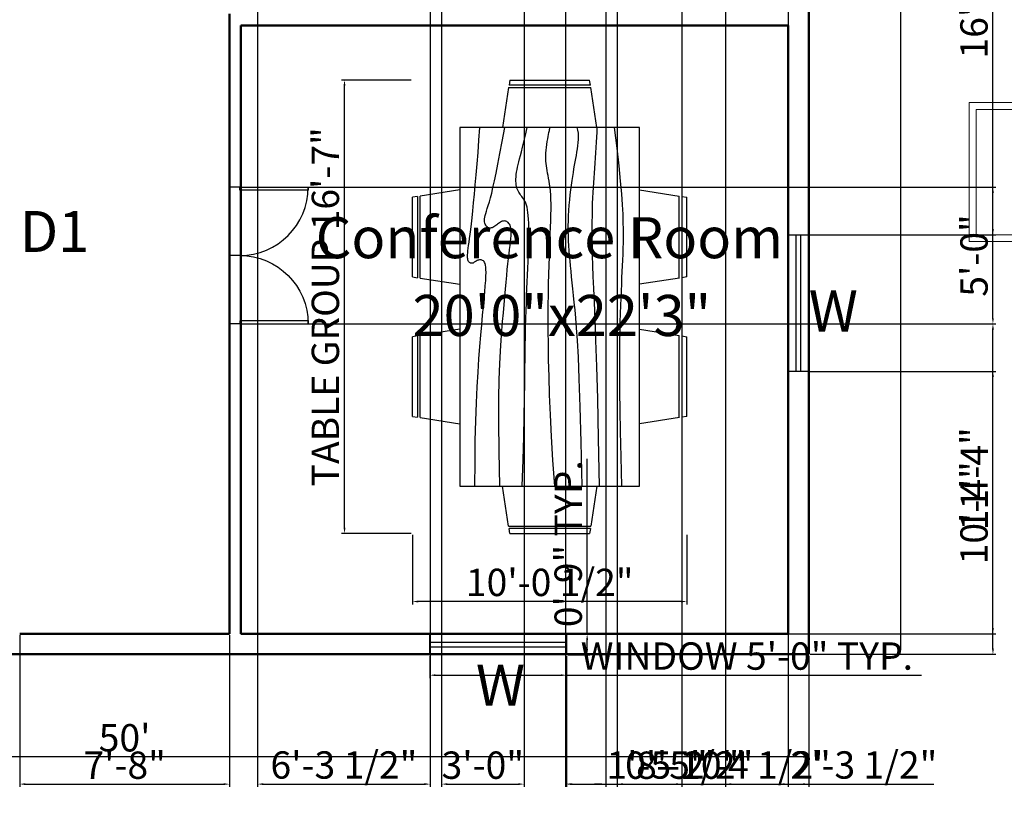
# Model space of a CAD drawing. Units: inches. Extents: x 1953 to 3378, y 1378 to 2530.
# Tile 2 of 5: x 2350 to 2782, y 1378 to 1725. Entities that reach past the tile are written whole.
import ezdxf

# ---------------------------------------------------------------- set-up
doc = ezdxf.new("R2010")
doc.units = ezdxf.units.IN
for name, color, linetype, lineweight in [('A-ANNO-DIMS', 2, 'Continuous', 18), ('A-ANNO-TEXT', 7, 'Continuous', 18), ('A-AREA-IDEN', 4, 'Continuous', 18), ('A-DOOR', 4, 'Continuous', 25), ('A-FURN', 50, 'Continuous', 25), ('wall', 7, 'Continuous', 50), ('windows', 180, 'Continuous', 25)]:
    doc.layers.add(name, color=color, linetype=linetype, lineweight=lineweight)
doc.styles.get("Standard").update_dxf_attribs({"font": 'arial.ttf'})
doc.dimstyles.new('ISO-25', dxfattribs={"dimtxt": 12, "dimasz": 2.5, "dimexe": 1.25, "dimexo": 0.625, "dimtad": 1, "dimdec": 1, "dimlunit": 4, "dimtxsty": 'Standard', "dimcen": 2.5, "dimadec": 0, "dimazin": 0, "dimtfac": 1, "dimtdec": 1, "dimtmove": 0, "dimatfit": 3, "dimfxl": 1, "dimarcsym": 0})

# ---------------------------------------------------------------- blocks, each defined once
blk = doc.blocks.new('*U2')
for p, q in [((0, 0), (0, -6)), ((40, 0), (40, -6))]:
    blk.add_line(p, q)
blk.add_lwpolyline([(0, 0), (0, 40), (1.75, 40), (1.75, 0)], close=True)
blk.add_arc((0, 0), 40, 0, 90)
blk = doc.blocks.new('Dining Set - 36 x 72 in.')
for p, q in [((-22.2343, 26.00059), (-23.4847, 17.99762)), ((-22.2304, 26), (-5.7608, 26)), ((-22, 27.5), (-22.1562, 26.50042)), ((-5.8416, 26.5), (-22.1534, 26.5)), ((-22, 27.5), (-6, 27.5)), ((-5.8437, 26.49966), (-6, 27.5)), ((-4.5152, 17.99762), (-5.7655, 25.99926)), ((5.7657, 26.00059), (4.5153, 17.99762)), ((5.7696, 26), (22.2392, 26)), ((6, 27.5), (5.8438, 26.50042)), ((22.1584, 26.5), (5.8466, 26.5)), ((6, 27.5), (22, 27.5)), ((22.1563, 26.49966), (22, 27.5)), ((23.4848, 17.99762), (22.2345, 25.99926)), ((36, 18), (-36, 18)), ((-36, 18), (-36, -18)), ((36, -18), (36, 18)), ((-45.5, 8), (-44.5004, 8.15617)), ((-45.5, 8), (-45.5, -8)), ((-44.5, -8.15843), (-44.5, 8.15338)), ((-44.0006, 8.23428), (-35.9976, 9.48474)), ((-44, 8.23041), (-44, -8.23915)), ((44.0006, 8.23428), (35.9976, 9.48474)), ((44, 8.23041), (44, -8.23915)), ((44.5, -8.15843), (44.5, 8.15338)), ((45.5, 8), (44.5005, 8.15617)), ((45.5, 8), (45.5, -8)), ((-44.4997, -8.15631), (-45.5, -8)), ((-35.9976, -9.48476), (-43.9993, -8.2345)), ((35.9976, -9.48476), (43.9993, -8.2345)), ((44.4997, -8.15631), (45.5, -8)), ((-36, -18), (36, -18)), ((-22.2343, -26.0006), (-23.4847, -17.99762)), ((-4.5152, -17.99762), (-5.7655, -25.99928)), ((5.7657, -26.0006), (4.5153, -17.99762)), ((23.4848, -17.99762), (22.2345, -25.99928)), ((-22.2304, -26), (-5.7608, -26)), ((-22, -27.5), (-22.1562, -26.50044)), ((-5.8416, -26.5), (-22.1534, -26.5)), ((-22, -27.5), (-6, -27.5)), ((-5.8437, -26.49967), (-6, -27.5)), ((5.7696, -26), (22.2392, -26)), ((6, -27.5), (5.8438, -26.50044)), ((22.1584, -26.5), (5.8466, -26.5)), ((6, -27.5), (22, -27.5)), ((22.1563, -26.49967), (22, -27.5))]:
    blk.add_line(p, q)
for points in [[(-36, 15), (-31.1772, 14.97754), (-26.8079, 14.91406), (-22.8538, 14.81543), (-19.276, 14.6875), (-16.0362, 14.53613), (-13.0957, 14.36718), (-10.4159, 14.18652), (-7.9583, 14), (-5.6904, 13.81315), (-3.6035, 13.63021), (-1.6954, 13.45508), (0.0365, 13.29166), (1.5945, 13.14388), (2.9811, 13.01562), (4.1988, 12.9108), (5.25, 12.83333), (6.1393, 12.78613), (6.8802, 12.76823), (7.4883, 12.77767), (7.9792, 12.8125), (8.3685, 12.87077), (8.6719, 12.95052), (8.9049, 13.0498), (9.0833, 13.16666), (9.2205, 13.29899), (9.3216, 13.44401), (9.3895, 13.59879), (9.4271, 13.76041), (9.4373, 13.92594), (9.4232, 14.09245), (9.3875, 14.257), (9.3333, 14.41666), (9.2638, 14.56917), (9.1836, 14.71484), (9.0975, 14.85465), (9.0104, 14.98958), (8.9272, 15.1206), (8.8529, 15.2487), (8.7922, 15.37483), (8.75, 15.5), (8.7305, 15.62467), (8.7344, 15.74739), (8.7617, 15.86621), (8.8125, 15.97916), (8.8867, 16.08431), (8.9844, 16.17968), (9.1055, 16.26334), (9.25, 16.33333), (9.4189, 16.38802), (9.6172, 16.42708), (9.8506, 16.45052), (10.125, 16.45833), (10.4463, 16.45052), (10.8203, 16.42708), (11.2529, 16.38802), (11.75, 16.33333), (12.3184, 16.26318), (12.9694, 16.17838), (13.7151, 16.07991), (14.5677, 15.96875), (15.5395, 15.84586), (16.6426, 15.71224), (17.8893, 15.56884), (19.2917, 15.41666), (20.859, 15.25667), (22.5879, 15.08984), (24.4721, 14.91715), (26.5052, 14.73958), (28.6809, 14.5581), (30.9929, 14.3737), (33.4347, 14.18733), (36, 14)], [(-36, 10), (-28.9766, 10.14274), (-23.1725, 10.20442), (-18.4241, 10.19775), (-14.5677, 10.13541), (-11.4399, 10.03011), (-8.877, 9.89453), (-6.7154, 9.74137), (-4.7917, 9.58333), (-2.9698, 9.43082), (-1.2246, 9.28515), (0.4415, 9.14534), (2.026, 9.01041), (3.5266, 8.87939), (4.9408, 8.7513), (6.266, 8.62516), (7.5, 8.5), (8.6411, 8.37549), (9.6914, 8.2539), (10.6538, 8.13818), (11.5312, 8.03125), (12.3267, 7.93603), (13.043, 7.85547), (13.6831, 7.79248), (14.25, 7.75), (14.7471, 7.7303), (15.1797, 7.73307), (15.5537, 7.75732), (15.875, 7.80208), (16.1494, 7.86637), (16.3828, 7.94922), (16.5811, 8.04964), (16.75, 8.16666), (16.8944, 8.29915), (17.0143, 8.44531), (17.1089, 8.60319), (17.1771, 8.77083), (17.218, 8.94629), (17.2305, 9.1276), (17.2137, 9.31282), (17.1667, 9.5), (17.0895, 9.6875), (16.987, 9.875), (16.8649, 10.0625), (16.7292, 10.25), (16.5856, 10.4375), (16.4401, 10.625), (16.2985, 10.8125), (16.1667, 11), (16.05, 11.18733), (15.9518, 11.3737), (15.8752, 11.5581), (15.8229, 11.73958), (15.798, 11.91715), (15.8034, 12.08984), (15.842, 12.25667), (15.9167, 12.41666), (16.0295, 12.56836), (16.1784, 12.70833), (16.3605, 12.83268), (16.5729, 12.9375), (16.8127, 13.01888), (17.0768, 13.07291), (17.3625, 13.0957), (17.6667, 13.08333), (17.9894, 13.03312), (18.3418, 12.94726), (18.7382, 12.82918), (19.1927, 12.68229), (19.7195, 12.51001), (20.3327, 12.31575), (21.0465, 12.10294), (21.875, 11.875), (22.8357, 11.63354), (23.959, 11.37304), (25.2786, 11.08618), (26.8282, 10.76562), (28.6414, 10.40405), (30.752, 9.99414), (33.1936, 9.52856), (36, 9)], [(-36, 5.5), (-30.7157, 5.3348), (-26.069, 5.20963), (-21.9946, 5.11767), (-18.4271, 5.05208), (-15.3009, 5.00602), (-12.5508, 4.97265), (-10.1112, 4.94515), (-7.9167, 4.91666), (-5.909, 4.88167), (-4.0586, 4.83984), (-2.3429, 4.79215), (-0.7396, 4.73958), (0.7739, 4.6831), (2.22, 4.6237), (3.6213, 4.56233), (5, 4.5), (6.373, 4.43782), (7.7344, 4.3776), (9.0723, 4.32129), (10.375, 4.27083), (11.6309, 4.22819), (12.8281, 4.19531), (13.9551, 4.17415), (15, 4.16666), (15.954, 4.17448), (16.819, 4.19791), (17.6001, 4.23698), (18.3021, 4.29166), (18.9299, 4.36198), (19.4883, 4.44791), (19.9823, 4.54948), (20.4167, 4.66666), (20.7969, 4.79899), (21.1302, 4.94401), (21.4245, 5.09879), (21.6875, 5.26041), (21.9271, 5.42594), (22.1511, 5.59245), (22.3672, 5.757), (22.5834, 5.91666), (22.8065, 6.06868), (23.0404, 6.21093), (23.2879, 6.34147), (23.5521, 6.45833), (23.8358, 6.55957), (24.142, 6.64323), (24.4735, 6.70735), (24.8334, 6.75), (25.2235, 6.76969), (25.642, 6.76692), (26.0858, 6.74267), (26.5521, 6.69791), (27.0379, 6.63362), (27.5404, 6.55078), (28.0565, 6.45036), (28.5834, 6.33333), (29.1242, 6.19987), (29.7071, 6.04687), (30.3661, 5.87044), (31.1354, 5.66666), (32.0493, 5.43164), (33.142, 5.16146), (34.4475, 4.85221), (36, 4.5)], [(-36, -1), (-30.7915, -0.6591), (-26.0195, -0.38216), (-21.6519, -0.16284), (-17.6563, 0.00521), (-14.0005, 0.12833), (-10.6523, 0.21289), (-7.5796, 0.26522), (-4.75, 0.29166), (-2.134, 0.29793), (0.2878, 0.28711), (2.5317, 0.26163), (4.6146, 0.22396), (6.5529, 0.17651), (8.3633, 0.12174), (10.0623, 0.06209), (11.6667, 0), (13.1899, -0.06201), (14.6341, -0.1211), (15.9982, -0.17432), (17.2813, -0.21875), (18.4823, -0.25147), (19.6003, -0.26953), (20.6343, -0.27002), (21.5834, -0.25), (22.4481, -0.20768), (23.2357, -0.14584), (23.9549, -0.06836), (24.6146, 0.02083), (25.2235, 0.11784), (25.7904, 0.21875), (26.3241, 0.31966), (26.8334, 0.41666), (27.3265, 0.50618), (27.8099, 0.58593), (28.2894, 0.65397), (28.7709, 0.70833), (29.2601, 0.74707), (29.763, 0.76823), (30.2855, 0.76985), (30.8334, 0.75), (31.4088, 0.70784), (31.9994, 0.64713), (32.589, 0.57275), (33.1615, 0.48958), (33.7008, 0.4025), (34.1908, 0.3164), (34.6153, 0.23616), (34.9584, 0.16666), (35.2099, 0.11165), (35.3848, 0.07031), (35.504, 0.04069), (35.5886, 0.02083), (35.6594, 0.00879), (35.7377, 0.0026), (35.8442, 0.00032), (36, 0)], [(-36, -6.5), (-27.1843, -6.31267), (-20.084, -6.1263), (-14.469, -5.9419), (-10.1094, -5.76042), (-6.7752, -5.58285), (-4.2363, -5.41016), (-2.2629, -5.24333), (-0.625, -5.08334), (0.8708, -4.93099), (2.2715, -4.78646), (3.5872, -4.64974), (4.8281, -4.52084), (6.0046, -4.39974), (7.127, -4.28646), (8.2053, -4.18099), (9.25, -4.08334), (10.2705, -3.99382), (11.2734, -3.91407), (12.2647, -3.84603), (13.25, -3.79167), (14.2354, -3.75293), (15.2266, -3.73177), (16.2295, -3.73015), (17.25, -3.75), (18.2912, -3.79248), (19.3451, -3.85547), (20.4009, -3.93604), (21.4479, -4.03125), (22.4754, -4.13819), (23.4727, -4.25391), (24.4289, -4.37549), (25.3334, -4.5), (26.1785, -4.62492), (26.9694, -4.74935), (27.7145, -4.87281), (28.4219, -4.99479), (29.1, -5.11483), (29.7572, -5.23242), (30.4016, -5.34709), (31.0417, -5.45834), (31.6837, -5.56437), (32.3262, -5.65821), (32.9658, -5.73153), (33.599, -5.77604), (34.2224, -5.78345), (34.8327, -5.74545), (35.4264, -5.65373), (36, -5.5)], [(-36, -10), (-26.4022, -9.81299), (-18.4675, -9.62891), (-11.9839, -9.45069), (-6.7396, -9.28125), (-2.5226, -9.12354), (0.8789, -8.98047), (3.6769, -8.85498), (6.0833, -8.75), (8.2767, -8.66765), (10.3021, -8.60677), (12.1712, -8.56543), (13.8958, -8.54167), (15.4876, -8.53353), (16.9583, -8.53907), (18.3197, -8.55632), (19.5834, -8.58334), (20.7616, -8.61841), (21.8685, -8.66081), (22.9188, -8.71004), (23.9271, -8.76563), (24.9081, -8.82707), (25.8763, -8.89388), (26.8465, -8.96558), (27.8334, -9.04167), (28.8474, -9.12118), (29.8828, -9.20117), (30.93, -9.27824), (31.9792, -9.34896), (33.0205, -9.40991), (34.0443, -9.45768), (35.0407, -9.48885), (36, -9.5)], [(-36, -14.5), (-30.0881, -14.33513), (-25.0332, -14.21224), (-20.7312, -14.12647), (-17.0781, -14.07292), (-13.97, -14.04671), (-11.3027, -14.04297), (-8.9724, -14.05681), (-6.875, -14.08334), (-4.9224, -14.11833), (-3.0905, -14.16016), (-1.3709, -14.20785), (0.2448, -14.26042), (1.7647, -14.3169), (3.1973, -14.3763), (4.5507, -14.43767), (5.8333, -14.5), (7.0554, -14.5621), (8.235, -14.62175), (9.3922, -14.67652), (10.5469, -14.72396), (11.7192, -14.76164), (12.929, -14.78711), (14.1965, -14.79794), (15.5417, -14.79167), (16.9933, -14.76424), (18.6152, -14.70508), (20.4804, -14.60197), (22.6615, -14.44271), (25.2312, -14.21509), (28.2624, -13.9069), (31.8277, -13.50594), (36, -13)]]:
    blk.add_lwpolyline(points)
blk = doc.blocks.new('*D27')
at = {"layer": 'A-ANNO-DIMS', "color": 0, "lineweight": -2, "transparency": 16777216}
for p, q in [((2696.37, 2286.01), (2737.23, 2286.01)), ((2735.98, 2283.51), (2735.98, 1448.51)), ((2696.37, 1446.01), (2737.23, 1446.01))]:
    blk.add_line(p, q, dxfattribs=at)
at = {"layer": 'A-ANNO-DIMS', "color": 0, "transparency": 16777216}
for points in [[(2735.56, 2283.51), (2736.4, 2283.51), (2735.98, 2286.01)], [(2735.56, 1448.51), (2736.4, 1448.51), (2735.98, 1446.01)]]:
    blk.add_solid(points, dxfattribs=at)
at = {"layer": 'Defpoints', "color": 0, "transparency": 16777216}
for p in [(2695.75, 2286.01), (2695.75, 1446.01), (2735.98, 1446.01)]:
    blk.add_point(p, dxfattribs=at)
at = {"layer": 'A-ANNO-DIMS', "color": 0, "transparency": 16777216, "insert": (2729.23, 1866.01), "char_height": 12, "attachment_point": 5, "rotation": 90}
blk.add_mtext("70'", dxfattribs=at)
blk = doc.blocks.new('*D28')
at = {"layer": 'A-ANNO-DIMS', "color": 0, "lineweight": -2, "transparency": 16777216}
for p, q in [((2095.75, 1445.39), (2095.75, 1399.8)), ((2695.75, 1445.39), (2695.75, 1399.8)), ((2693.25, 1401.05), (2098.25, 1401.05))]:
    blk.add_line(p, q, dxfattribs=at)
at = {"layer": 'A-ANNO-DIMS', "color": 0, "transparency": 16777216}
for points in [[(2098.25, 1401.47), (2098.25, 1400.63), (2095.75, 1401.05)], [(2693.25, 1401.47), (2693.25, 1400.63), (2695.75, 1401.05)]]:
    blk.add_solid(points, dxfattribs=at)
at = {"layer": 'Defpoints', "color": 0, "transparency": 16777216}
for p in [(2095.75, 1446.01), (2695.75, 1446.01), (2095.75, 1401.05)]:
    blk.add_point(p, dxfattribs=at)
at = {"layer": 'A-ANNO-DIMS', "color": 0, "transparency": 16777216, "insert": (2395.75, 1407.8), "char_height": 12, "attachment_point": 5}
blk.add_mtext("50'", dxfattribs=at)
blk = doc.blocks.new('WINDOW-60IN')
for p, q in [((0, 5.5), (60, 5.5)), ((0, 5.5), (60, 5.5)), ((0, 3.5), (60, 3.5))]:
    blk.add_line(p, q)
blk.add_lwpolyline([(0, 9), (60, 9), (60, 0), (0, 0)], close=True)
blk = doc.blocks.new('*D38')
at = {"layer": 'A-ANNO-DIMS', "color": 0, "lineweight": -2, "transparency": 16777216}
for p, q in [((2529.57, 1445.21), (2529.57, 1435.58)), ((2589.57, 1445.21), (2589.57, 1435.58)), ((2532.07, 1436.83), (2587.07, 1436.83)), ((2589.57, 1436.83), (2745.17, 1436.83))]:
    blk.add_line(p, q, dxfattribs=at)
at = {"layer": 'A-ANNO-DIMS', "color": 0, "transparency": 16777216}
for points in [[(2532.07, 1437.25), (2532.07, 1436.42), (2529.57, 1436.83)], [(2587.07, 1437.25), (2587.07, 1436.42), (2589.57, 1436.83)]]:
    blk.add_solid(points, dxfattribs=at)
at = {"layer": 'Defpoints', "color": 0, "transparency": 16777216}
for p in [(2529.57, 1445.83), (2589.57, 1445.83), (2589.57, 1436.83)]:
    blk.add_point(p, dxfattribs=at)
at = {"layer": 'A-ANNO-DIMS', "color": 0, "transparency": 16777216, "insert": (2668.62, 1443.67), "char_height": 12, "attachment_point": 5}
blk.add_mtext('WINDOW 5\'-0" TYP.', dxfattribs=at)
blk = doc.blocks.new('*D39')
at = {"layer": 'A-ANNO-DIMS', "color": 0, "lineweight": -2, "transparency": 16777216}
for p, q in [((2598.57, 1454.83), (2598.57, 1531.73)), ((2590.19, 1454.83), (2599.82, 1454.83)), ((2598.57, 1448.33), (2598.57, 1452.33)), ((2590.19, 1445.83), (2599.82, 1445.83))]:
    blk.add_line(p, q, dxfattribs=at)
at = {"layer": 'A-ANNO-DIMS', "color": 0, "transparency": 16777216}
for points in [[(2598.15, 1452.33), (2598.98, 1452.33), (2598.57, 1454.83)], [(2598.15, 1448.33), (2598.98, 1448.33), (2598.57, 1445.83)]]:
    blk.add_solid(points, dxfattribs=at)
at = {"layer": 'Defpoints', "color": 0, "transparency": 16777216}
for p in [(2589.57, 1454.83), (2598.57, 1454.83), (2589.57, 1445.83)]:
    blk.add_point(p, dxfattribs=at)
at = {"layer": 'A-ANNO-DIMS', "color": 0, "transparency": 16777216, "insert": (2591.82, 1494.53), "char_height": 12, "attachment_point": 5, "rotation": 90}
blk.add_mtext('0\'-9" TYP.', dxfattribs=at)
blk = doc.blocks.new('*D50')
at = {"layer": 'A-ANNO-DIMS', "color": 0, "lineweight": -2, "transparency": 16777216}
for p, q in [((2521.4, 1697.99), (2490.93, 1697.99)), ((2492.18, 1501.51), (2492.18, 1695.49)), ((2521.4, 1499.01), (2490.93, 1499.01))]:
    blk.add_line(p, q, dxfattribs=at)
at = {"layer": 'A-ANNO-DIMS', "color": 0, "transparency": 16777216}
for points in [[(2491.76, 1695.49), (2492.59, 1695.49), (2492.18, 1697.99)], [(2491.76, 1501.51), (2492.59, 1501.51), (2492.18, 1499.01)]]:
    blk.add_solid(points, dxfattribs=at)
at = {"layer": 'Defpoints', "color": 0, "transparency": 16777216}
for p in [(2492.18, 1697.99), (2522.02, 1697.99), (2522.02, 1499.01)]:
    blk.add_point(p, dxfattribs=at)
at = {"layer": 'A-ANNO-DIMS', "color": 0, "transparency": 16777216, "insert": (2485.34, 1598.5), "char_height": 12, "attachment_point": 5, "rotation": 90}
blk.add_mtext('TABLE GROUP 16\'-7"', dxfattribs=at)
blk = doc.blocks.new('*D51')
at = {"layer": 'A-ANNO-DIMS', "color": 0, "lineweight": -2, "transparency": 16777216}
for p, q in [((2522.02, 1498.39), (2522.02, 1467.92)), ((2642.28, 1498.39), (2642.28, 1467.92)), ((2639.78, 1469.17), (2524.52, 1469.17))]:
    blk.add_line(p, q, dxfattribs=at)
at = {"layer": 'A-ANNO-DIMS', "color": 0, "transparency": 16777216}
for points in [[(2524.52, 1469.59), (2524.52, 1468.75), (2522.02, 1469.17)], [(2639.78, 1469.59), (2639.78, 1468.75), (2642.28, 1469.17)]]:
    blk.add_solid(points, dxfattribs=at)
at = {"layer": 'Defpoints', "color": 0, "transparency": 16777216}
for p in [(2522.02, 1499.01), (2642.28, 1499.01), (2522.02, 1469.17)]:
    blk.add_point(p, dxfattribs=at)
at = {"layer": 'A-ANNO-DIMS', "color": 0, "transparency": 16777216, "insert": (2582.15, 1476), "char_height": 12, "attachment_point": 5}
blk.add_mtext('10\'-0 1/2"', dxfattribs=at)
blk = doc.blocks.new('*D70')
at = {"layer": 'A-ANNO-DIMS', "color": 0, "lineweight": -2, "transparency": 16777216}
for p, q in [((2696.37, 1570.16), (2777.76, 1570.16)), ((2776.51, 1448.51), (2776.51, 1567.66)), ((2696.37, 1446.01), (2777.76, 1446.01))]:
    blk.add_line(p, q, dxfattribs=at)
at = {"layer": 'A-ANNO-DIMS', "color": 0, "transparency": 16777216}
for points in [[(2776.09, 1567.66), (2776.93, 1567.66), (2776.51, 1570.16)], [(2776.09, 1448.51), (2776.93, 1448.51), (2776.51, 1446.01)]]:
    blk.add_solid(points, dxfattribs=at)
at = {"layer": 'Defpoints', "color": 0, "transparency": 16777216}
for p in [(2695.75, 1570.16), (2776.51, 1570.16), (2695.75, 1446.01)]:
    blk.add_point(p, dxfattribs=at)
at = {"layer": 'A-ANNO-DIMS', "color": 0, "transparency": 16777216, "insert": (2769.76, 1508.09), "char_height": 12, "attachment_point": 5, "rotation": 90}
blk.add_mtext('10\'-4"', dxfattribs=at)
blk = doc.blocks.new('*D71')
at = {"layer": 'A-ANNO-DIMS', "color": 0, "lineweight": -2, "transparency": 16777216}
for p, q in [((2589.57, 1445.21), (2589.57, 1387.78)), ((2695.75, 1445.39), (2695.75, 1387.78)), ((2592.07, 1389.03), (2693.25, 1389.03))]:
    blk.add_line(p, q, dxfattribs=at)
at = {"layer": 'A-ANNO-DIMS', "color": 0, "transparency": 16777216}
for points in [[(2592.07, 1389.45), (2592.07, 1388.62), (2589.57, 1389.03)], [(2693.25, 1389.45), (2693.25, 1388.62), (2695.75, 1389.03)]]:
    blk.add_solid(points, dxfattribs=at)
at = {"layer": 'Defpoints', "color": 0, "transparency": 16777216}
for p in [(2589.57, 1445.83), (2695.75, 1446.01), (2695.75, 1389.03)]:
    blk.add_point(p, dxfattribs=at)
at = {"layer": 'A-ANNO-DIMS', "color": 0, "transparency": 16777216, "insert": (2642.66, 1395.79), "char_height": 12, "attachment_point": 5}
blk.add_mtext('8\'-10"', dxfattribs=at)
blk = doc.blocks.new('*D72')
at = {"layer": 'A-ANNO-DIMS', "color": 0, "lineweight": -2, "transparency": 16777216}
for p, q in [((2696.37, 1830.01), (2777.76, 1830.01)), ((2776.51, 1632.66), (2776.51, 1827.51)), ((2696.37, 1630.16), (2777.76, 1630.16))]:
    blk.add_line(p, q, dxfattribs=at)
at = {"layer": 'A-ANNO-DIMS', "color": 0, "transparency": 16777216}
for points in [[(2776.09, 1827.51), (2776.93, 1827.51), (2776.51, 1830.01)], [(2776.09, 1632.66), (2776.93, 1632.66), (2776.51, 1630.16)]]:
    blk.add_solid(points, dxfattribs=at)
at = {"layer": 'Defpoints', "color": 0, "transparency": 16777216}
for p in [(2695.75, 1830.01), (2776.51, 1830.01), (2695.75, 1630.16)]:
    blk.add_point(p, dxfattribs=at)
at = {"layer": 'A-ANNO-DIMS', "color": 0, "transparency": 16777216, "insert": (2769.76, 1730.09), "char_height": 12, "attachment_point": 5, "rotation": 90}
blk.add_mtext('16\'-8"', dxfattribs=at)
blk = doc.blocks.new('*D74')
at = {"layer": 'A-ANNO-DIMS', "color": 0, "lineweight": -2, "transparency": 16777216}
for p, q in [((2454.07, 2276.39), (2454.07, 1387.78)), ((2529.75, 2276.39), (2529.75, 1387.78)), ((2456.57, 1389.03), (2527.25, 1389.03))]:
    blk.add_line(p, q, dxfattribs=at)
at = {"layer": 'A-ANNO-DIMS', "color": 0, "transparency": 16777216}
for points in [[(2456.57, 1389.45), (2456.57, 1388.62), (2454.07, 1389.03)], [(2527.25, 1389.45), (2527.25, 1388.62), (2529.75, 1389.03)]]:
    blk.add_solid(points, dxfattribs=at)
at = {"layer": 'Defpoints', "color": 0, "transparency": 16777216}
for p in [(2454.07, 2277.01), (2529.75, 2277.01), (2529.75, 1389.03)]:
    blk.add_point(p, dxfattribs=at)
at = {"layer": 'A-ANNO-DIMS', "color": 0, "transparency": 16777216, "insert": (2491.91, 1395.87), "char_height": 12, "attachment_point": 5}
blk.add_mtext('6\'-3 1/2"', dxfattribs=at)
blk = doc.blocks.new('*D75')
at = {"layer": 'A-ANNO-DIMS', "color": 0, "lineweight": -2, "transparency": 16777216}
for p, q in [((2446.87, 1651.01), (2777.76, 1651.01)), ((2776.51, 1593.51), (2776.51, 1648.51)), ((2446.87, 1591.01), (2777.76, 1591.01))]:
    blk.add_line(p, q, dxfattribs=at)
at = {"layer": 'A-ANNO-DIMS', "color": 0, "transparency": 16777216}
for points in [[(2776.09, 1648.51), (2776.93, 1648.51), (2776.51, 1651.01)], [(2776.09, 1593.51), (2776.93, 1593.51), (2776.51, 1591.01)]]:
    blk.add_solid(points, dxfattribs=at)
at = {"layer": 'Defpoints', "color": 0, "transparency": 16777216}
for p in [(2446.25, 1651.01), (2776.51, 1651.01), (2446.25, 1591.01)]:
    blk.add_point(p, dxfattribs=at)
at = {"layer": 'A-ANNO-DIMS', "color": 0, "transparency": 16777216, "insert": (2769.76, 1621.01), "char_height": 12, "attachment_point": 5, "rotation": 90}
blk.add_mtext('5\'-0"', dxfattribs=at)
blk = doc.blocks.new('*D76')
at = {"layer": 'A-ANNO-DIMS', "color": 0, "lineweight": -2, "transparency": 16777216}
for p, q in [((2349.75, 1454.39), (2349.75, 1387.78)), ((2441.75, 1454.39), (2441.75, 1387.78)), ((2352.25, 1389.03), (2439.25, 1389.03))]:
    blk.add_line(p, q, dxfattribs=at)
at = {"layer": 'A-ANNO-DIMS', "color": 0, "transparency": 16777216}
for points in [[(2352.25, 1389.45), (2352.25, 1388.62), (2349.75, 1389.03)], [(2439.25, 1389.45), (2439.25, 1388.62), (2441.75, 1389.03)]]:
    blk.add_solid(points, dxfattribs=at)
at = {"layer": 'Defpoints', "color": 0, "transparency": 16777216}
for p in [(2349.75, 1455.01), (2441.75, 1455.01), (2441.75, 1389.03)]:
    blk.add_point(p, dxfattribs=at)
at = {"layer": 'A-ANNO-DIMS', "color": 0, "transparency": 16777216, "insert": (2395.75, 1395.79), "char_height": 12, "attachment_point": 5}
blk.add_mtext('7\'-8"', dxfattribs=at)
blk = doc.blocks.new('*D77')
at = {"layer": 'A-ANNO-DIMS', "color": 0, "lineweight": -2, "transparency": 16777216}
for p, q in [((2446.87, 1591.01), (2777.76, 1591.01)), ((2776.51, 1457.51), (2776.51, 1588.51)), ((2447.37, 1455.01), (2777.76, 1455.01))]:
    blk.add_line(p, q, dxfattribs=at)
at = {"layer": 'A-ANNO-DIMS', "color": 0, "transparency": 16777216}
for points in [[(2776.09, 1588.51), (2776.93, 1588.51), (2776.51, 1591.01)], [(2776.09, 1457.51), (2776.93, 1457.51), (2776.51, 1455.01)]]:
    blk.add_solid(points, dxfattribs=at)
at = {"layer": 'Defpoints', "color": 0, "transparency": 16777216}
for p in [(2446.25, 1591.01), (2776.51, 1591.01), (2446.75, 1455.01)]:
    blk.add_point(p, dxfattribs=at)
at = {"layer": 'A-ANNO-DIMS', "color": 0, "transparency": 16777216, "insert": (2769.86, 1523.01), "char_height": 12, "attachment_point": 5, "rotation": 90}
blk.add_mtext('11\'-4"', dxfattribs=at)
blk = doc.blocks.new('*D80')
at = {"layer": 'A-ANNO-DIMS', "color": 0, "lineweight": -2, "transparency": 16777216}
for p, q in [((2534.75, 2161.39), (2534.75, 1387.78)), ((2570.9, 2161.44), (2570.9, 1387.78)), ((2537.25, 1389.03), (2568.4, 1389.03))]:
    blk.add_line(p, q, dxfattribs=at)
at = {"layer": 'A-ANNO-DIMS', "color": 0, "transparency": 16777216}
for points in [[(2537.25, 1389.45), (2537.25, 1388.62), (2534.75, 1389.03)], [(2568.4, 1389.45), (2568.4, 1388.62), (2570.9, 1389.03)]]:
    blk.add_solid(points, dxfattribs=at)
at = {"layer": 'Defpoints', "color": 0, "transparency": 16777216}
for p in [(2534.75, 2162.01), (2570.9, 2162.07), (2570.9, 1389.03)]:
    blk.add_point(p, dxfattribs=at)
at = {"layer": 'A-ANNO-DIMS', "color": 0, "transparency": 16777216, "insert": (2552.82, 1395.79), "char_height": 12, "attachment_point": 5}
blk.add_mtext('3\'-0"', dxfattribs=at)
blk = doc.blocks.new('*D81')
at = {"layer": 'A-ANNO-DIMS', "color": 0, "lineweight": -2, "transparency": 16777216}
for p, q in [((2659.25, 2159.09), (2659.25, 1387.78)), ((2686.75, 2161.39), (2686.75, 1387.78)), ((2661.75, 1389.03), (2684.25, 1389.03)), ((2686.75, 1389.03), (2750.56, 1389.03))]:
    blk.add_line(p, q, dxfattribs=at)
at = {"layer": 'A-ANNO-DIMS', "color": 0, "transparency": 16777216}
for points in [[(2661.75, 1389.45), (2661.75, 1388.62), (2659.25, 1389.03)], [(2684.25, 1389.45), (2684.25, 1388.62), (2686.75, 1389.03)]]:
    blk.add_solid(points, dxfattribs=at)
at = {"layer": 'Defpoints', "color": 0, "transparency": 16777216}
for p in [(2659.25, 2159.71), (2686.75, 2162.01), (2686.75, 1389.03)]:
    blk.add_point(p, dxfattribs=at)
at = {"layer": 'A-ANNO-DIMS', "color": 0, "transparency": 16777216, "insert": (2719.91, 1395.87), "char_height": 12, "attachment_point": 5}
blk.add_mtext('2\'-3 1/2"', dxfattribs=at)
blk = doc.blocks.new('*D82')
at = {"layer": 'A-ANNO-DIMS', "color": 0, "lineweight": -2, "transparency": 16777216}
for p, q in [((2606.75, 2161.39), (2606.75, 1387.78)), ((2611.75, 2161.39), (2611.75, 1387.78)), ((2604.25, 1389.03), (2601.75, 1389.03)), ((2606.75, 1389.03), (2611.75, 1389.03)), ((2614.25, 1389.03), (2649.9, 1389.03))]:
    blk.add_line(p, q, dxfattribs=at)
at = {"layer": 'A-ANNO-DIMS', "color": 0, "transparency": 16777216}
for points in [[(2604.25, 1389.45), (2604.25, 1388.62), (2606.75, 1389.03)], [(2614.25, 1389.45), (2614.25, 1388.62), (2611.75, 1389.03)]]:
    blk.add_solid(points, dxfattribs=at)
at = {"layer": 'Defpoints', "color": 0, "transparency": 16777216}
for p in [(2606.75, 2162.01), (2611.75, 2162.01), (2611.75, 1389.03)]:
    blk.add_point(p, dxfattribs=at)
at = {"layer": 'A-ANNO-DIMS', "color": 0, "transparency": 16777216, "insert": (2633.32, 1395.79), "char_height": 12, "attachment_point": 5}
blk.add_mtext('0\'-5"', dxfattribs=at)
blk = doc.blocks.new('*D84')
at = {"layer": 'A-ANNO-DIMS', "color": 0, "lineweight": -2, "transparency": 16777216}
for p, q in [((2606.75, 2276.39), (2606.75, 1387.78)), ((2589.14, 2267.41), (2589.14, 1387.78)), ((2591.64, 1389.03), (2604.25, 1389.03)), ((2606.75, 1389.03), (2669.23, 1389.03))]:
    blk.add_line(p, q, dxfattribs=at)
at = {"layer": 'A-ANNO-DIMS', "color": 0, "transparency": 16777216}
for points in [[(2591.64, 1389.45), (2591.64, 1388.62), (2589.14, 1389.03)], [(2604.25, 1389.45), (2604.25, 1388.62), (2606.75, 1389.03)]]:
    blk.add_solid(points, dxfattribs=at)
at = {"layer": 'Defpoints', "color": 0, "transparency": 16777216}
for p in [(2606.75, 2277.01), (2589.14, 2268.03), (2606.75, 1389.03)]:
    blk.add_point(p, dxfattribs=at)
at = {"layer": 'A-ANNO-DIMS', "color": 0, "transparency": 16777216, "insert": (2639.24, 1395.86), "char_height": 12, "attachment_point": 5}
blk.add_mtext('1\'-5 1/2"', dxfattribs=at)
blk = doc.blocks.new('*D85')
at = {"layer": 'A-ANNO-DIMS', "color": 0, "lineweight": -2, "transparency": 16777216}
for p, q in [((2611.75, 2276.39), (2611.75, 1387.78)), ((2640.05, 2268.38), (2640.05, 1387.78)), ((2614.25, 1389.03), (2637.55, 1389.03)), ((2640.05, 1389.03), (2703.87, 1389.03))]:
    blk.add_line(p, q, dxfattribs=at)
at = {"layer": 'A-ANNO-DIMS', "color": 0, "transparency": 16777216}
for points in [[(2614.25, 1389.45), (2614.25, 1388.62), (2611.75, 1389.03)], [(2637.55, 1389.45), (2637.55, 1388.62), (2640.05, 1389.03)]]:
    blk.add_solid(points, dxfattribs=at)
at = {"layer": 'Defpoints', "color": 0, "transparency": 16777216}
for p in [(2611.75, 2277.01), (2640.05, 2269), (2640.05, 1389.03)]:
    blk.add_point(p, dxfattribs=at)
at = {"layer": 'A-ANNO-DIMS', "color": 0, "transparency": 16777216, "insert": (2673.21, 1395.86), "char_height": 12, "attachment_point": 5}
blk.add_mtext('2\'-4 1/2"', dxfattribs=at)

msp = doc.modelspace()

# ---------------------------------------------------------------- linework, layer by layer
at = {"layer": 'A-ANNO-TEXT'}
for points in [[(2766.11, 1688.1), (3378.35, 1688.1), (3378.35, 1627.13), (2766.11, 1627.13)], [(2769.11, 1685.1), (3375.35, 1685.1), (3375.35, 1630.13), (2769.11, 1630.13)]]:
    msp.add_lwpolyline(points, close=True, dxfattribs=at)
at = {"layer": 'wall'}
for p, q in [((2695.75, 2286.01), (2695.75, 1446.01)), ((2441.75, 1727.01), (2441.75, 1455.01)), ((2446.75, 1722.01), (2446.75, 1455.01)), ((2446.75, 1722.01), (2686.75, 1722.01)), ((2686.75, 1722.01), (2686.75, 1650.01)), ((2686.75, 1722.01), (2686.75, 1455.01)), ((2441.75, 1455.01), (2349.75, 1455.01)), ((2686.75, 1455.01), (2446.75, 1455.01)), ((2695.75, 1446.01), (2095.75, 1446.01))]:
    msp.add_line(p, q, dxfattribs=at)

# ---------------------------------------------------------------- block references
at = {"layer": 'A-DOOR', "yscale": 0.75, "zscale": 0.75, "rotation": 270}
for p, xscale in [((2446.25, 1651.01), 0.75), ((2446.25, 1591.01), -0.75)]:
    msp.add_blockref('*U2', p, dxfattribs=dict(at, xscale=xscale))
at = {"layer": 'A-FURN', "xscale": 2.186505354454292, "yscale": 2.186505354454292, "zscale": 2.186505354454292, "rotation": 89.99999999999999}
msp.add_blockref('Dining Set - 36 x 72 in.', (2582.15, 1598.5), dxfattribs=at)
at = {"layer": 'windows', "rotation": 90.00000000000072}
msp.add_blockref('WINDOW-60IN', (2695.75, 1570.16), dxfattribs=at)
at = {"layer": 'windows'}
msp.add_blockref('WINDOW-60IN', (2529.57, 1445.83), dxfattribs=at)

# ---------------------------------------------------------------- texts
at = {"layer": 'A-ANNO-TEXT'}
for s, p in [('D1', (2349.75, 1622.56)), ('W', (2695.75, 1587.66)), ('W', (2549.79, 1423.41))]:
    msp.add_text(s, height=18, dxfattribs=at).set_placement(p)
at = {"layer": 'A-AREA-IDEN'}
for s, p in [('Conference Room', (2479.54, 1619.83)), ('20\'0"x22\'3"', (2522.02, 1585.7))]:
    msp.add_text(s, height=18, dxfattribs=at).set_placement(p)

# ---------------------------------------------------------------- dimensions: what is measured, and where the dimension line sits
at = {"layer": 'A-ANNO-DIMS'}
for base, p1, p2, angle, override, picture, middle in [((2735.98, 1446.01), (2695.75, 2286.01), (2695.75, 1446.01), 90, {"dimclrd": 0, "dimclre": 0, "dimclrt": 0}, '*D27', (2729.23, 1866.01)), ((2776.5098, 1830.0108), (2695.7476, 1630.1645), (2695.7476, 1830.0108), 90, {"dimdec": 1, "dimlfac": 1, "dimrnd": 0, "dimzin": 1, "dimdsep": 46, "dimlunit": 4, "dimfrac": 2}, '*D72', (2769.758, 1730.0877)), ((2776.51, 1651.01), (2446.25, 1591.01), (2446.25, 1651.01), 90, {"dimdec": 1, "dimlfac": 1, "dimrnd": 0, "dimzin": 1, "dimdsep": 46, "dimlunit": 4, "dimfrac": 2}, '*D75', (2769.76, 1621.01)), ((2776.51, 1591.01), (2446.75, 1455.01), (2446.25, 1591.01), 90, {"dimdec": 1, "dimlfac": 1, "dimrnd": 0, "dimzin": 1, "dimdsep": 46, "dimlunit": 4, "dimfrac": 2}, '*D77', (2769.86, 1523.01)), ((2776.5098, 1570.1645), (2695.7476, 1446.0108), (2695.7476, 1570.1645), 90, {"dimdec": 1, "dimlfac": 1, "dimrnd": 0, "dimzin": 1, "dimdsep": 46, "dimlunit": 4, "dimfrac": 2}, '*D70', (2769.758, 1508.0877)), ((2522.02, 1469.17), (2642.28, 1499.01), (2522.02, 1499.01), 180, {"dimdec": 1, "dimlfac": 1, "dimrnd": 0, "dimzin": 1, "dimdsep": 46, "dimlunit": 4, "dimfrac": 2}, '*D51', (2582.15, 1476))]:
    dim = msp.add_linear_dim(base=base, p1=p1, p2=p2, angle=angle, dimstyle='ISO-25', override=override, dxfattribs=at)
    dim.commit()
    dim.dimension.update_dxf_attribs({"geometry": picture, "text_midpoint": middle})
for base, p1, p2, override, picture, middle in [((2529.75, 1389.03), (2454.07, 2277.01), (2529.75, 2277.01), {"dimdec": 1, "dimlfac": 1, "dimrnd": 0, "dimzin": 1, "dimdsep": 46, "dimlunit": 4, "dimfrac": 2}, '*D74', (2491.91, 1395.87)), ((2606.75, 1389.03), (2589.14, 2268.03), (2606.75, 2277.01), {"dimdec": 1, "dimlfac": 1, "dimrnd": 0, "dimzin": 1, "dimdsep": 46, "dimlunit": 4, "dimfrac": 2}, '*D84', (2639.24, 1395.86)), ((2640.05, 1389.03), (2611.75, 2277.01), (2640.05, 2269), {"dimdec": 1, "dimlfac": 1, "dimrnd": 0, "dimzin": 1, "dimdsep": 46, "dimlunit": 4, "dimfrac": 2}, '*D85', (2673.21, 1395.86)), ((2570.9022, 1389.0336), (2534.7476, 2162.0108), (2570.9022, 2162.0653), {"dimdec": 1, "dimlfac": 1, "dimrnd": 0, "dimzin": 1, "dimdsep": 46, "dimlunit": 4, "dimfrac": 2}, '*D80', (2552.8249, 1395.7895)), ((2611.75, 1389.03), (2606.75, 2162.01), (2611.75, 2162.01), {"dimdec": 1, "dimlfac": 1, "dimrnd": 0, "dimzin": 1, "dimdsep": 46, "dimlunit": 4, "dimfrac": 2}, '*D82', (2633.32, 1395.79)), ((2686.75, 1389.03), (2659.25, 2159.71), (2686.75, 2162.01), {"dimdec": 1, "dimlfac": 1, "dimrnd": 0, "dimzin": 1, "dimdsep": 46, "dimlunit": 4, "dimfrac": 2}, '*D81', (2719.91, 1395.87)), ((2441.75, 1389.03), (2349.75, 1455.01), (2441.75, 1455.01), {"dimdec": 1, "dimlfac": 1, "dimrnd": 0, "dimzin": 1, "dimdsep": 46, "dimlunit": 4, "dimfrac": 2}, '*D76', (2395.75, 1395.79)), ((2095.75, 1401.05), (2695.75, 1446.01), (2095.75, 1446.01), {"dimclrd": 0, "dimclre": 0, "dimclrt": 0}, '*D28', (2395.75, 1407.8)), ((2695.75, 1389.03), (2589.57, 1445.83), (2695.75, 1446.01), {"dimdec": 1, "dimlfac": 1, "dimrnd": 0, "dimzin": 1, "dimdsep": 46, "dimlunit": 4, "dimfrac": 2}, '*D71', (2642.66, 1395.79))]:
    dim = msp.add_linear_dim(base=base, p1=p1, p2=p2, dimstyle='ISO-25', override=override, dxfattribs=at)
    dim.commit()
    dim.dimension.update_dxf_attribs({"geometry": picture, "text_midpoint": middle})
for base, p1, p2, text, picture, middle in [((2492.18, 1697.99), (2522.02, 1499.01), (2522.02, 1697.99), 'TABLE GROUP <>', '*D50', (2485.34, 1598.5)), ((2598.57, 1454.83), (2589.57, 1445.83), (2589.57, 1454.83), '<> TYP.', '*D39', (2591.82, 1494.53))]:
    dim = msp.add_linear_dim(base=base, p1=p1, p2=p2, angle=90, text=text, dimstyle='ISO-25', override={"dimdec": 1, "dimlfac": 1, "dimrnd": 0, "dimzin": 1, "dimdsep": 46, "dimlunit": 4, "dimfrac": 2}, dxfattribs=at)
    dim.commit()
    dim.dimension.update_dxf_attribs({"geometry": picture, "text_midpoint": middle})
dim = msp.add_linear_dim(base=(2589.57, 1436.83), p1=(2529.57, 1445.83), p2=(2589.57, 1445.83), text='WINDOW <> TYP.', dimstyle='ISO-25', override={"dimdec": 1, "dimlfac": 1, "dimrnd": 0, "dimzin": 1, "dimdsep": 46, "dimlunit": 4, "dimfrac": 2}, dxfattribs=at)
dim.commit()
dim.dimension.update_dxf_attribs({"geometry": '*D38', "text_midpoint": (2668.62, 1443.67)})

doc.saveas('drawing.dxf')
